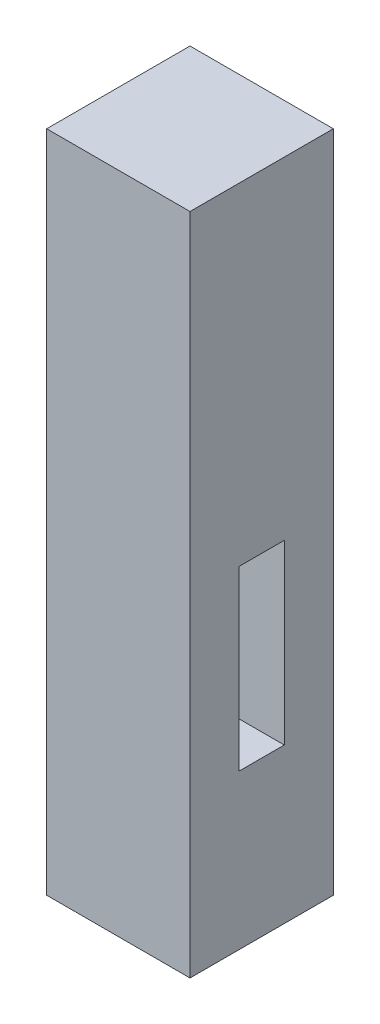
SolidWorks part; units mm, degrees
material "Plain Carbon Steel"
ref_plane "Front Plane" through (0, 0, 0) normal (0, 0, 1) x (1, 0, 0)
ref_plane "Top Plane" through (0, 0, 0) normal (0, 1, 0) x (1, 0, 0)
ref_plane "Right Plane" through (0, 0, 0) normal (1, 0, 0) x (0, 0, -1)
sketch "Rod Section Sketch 38x38" plane through (0, 0, 0) normal (0, 1, 0) x (1, 0, 0)
  line L1 (-19, -19) -> (19, -19)
  line L2 (-19, -19) -> (-19, 19)
  line L3 (-19, 19) -> (19, 19)
  line L4 (19, -19) -> (19, 19)
  line L5 (-19, -19) -> (19, 19) construction
  line L6 (-19, 19) -> (19, -19) construction
  point P0 (0, 0)
  dimension "D1" = 38
  dimension "D2" = 38
extrude "Square Rod 38x38x176" add sketch "Rod Section Sketch 38x38" along normal blind 176
sketch "Slot Profile Sketch" plane through (19, 0, 0) normal (1, 0, 0) x (0, 0, -1)
  line L0 (-19, 0) -> (19, 0) construction
  line L1 (-6, 41) -> (6, 41)
  line L2 (-6, 41) -> (-6, 88)
  line L3 (-6, 88) -> (6, 88)
  line L4 (6, 41) -> (6, 88)
  line L5 (-6, 41) -> (6, 88) construction
  line L6 (-6, 88) -> (6, 41) construction
  point P0 (0, 64.5)
  dimension "D1" = 47
  dimension "D2" = 41
  dimension "D3" = 12
extrude "Through Slot 47x12" cut sketch "Slot Profile Sketch" against normal blind 176
